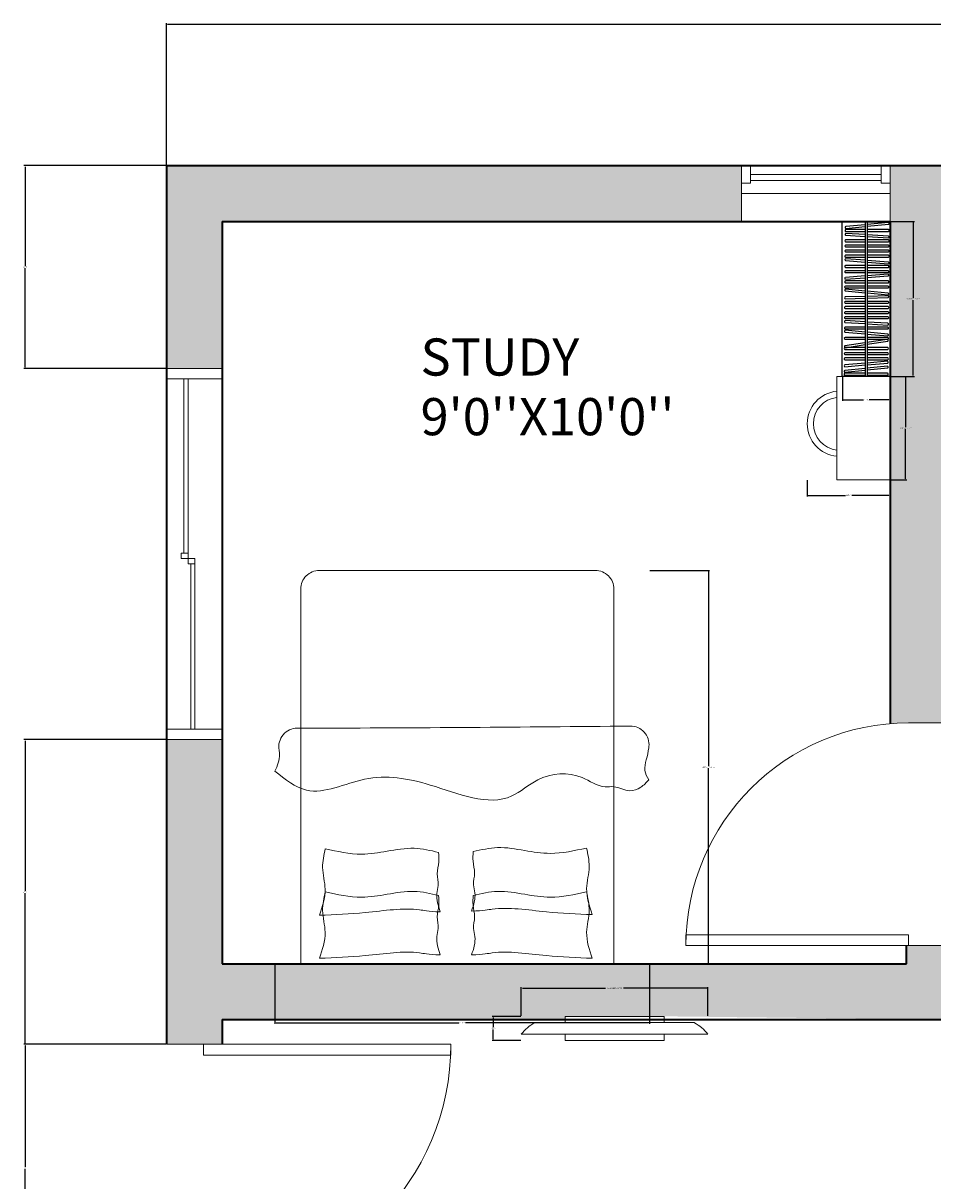
# Model space of a CAD drawing. Units: inches. Extents: x 1789 to 2841, y 3180 to 3702.
# Tile 12 of 14: x 2374 to 2521, y 3491 to 3678. Entities that reach past the tile are written whole.
import ezdxf

# ---------------------------------------------------------------- set-up
doc = ezdxf.new("R2010")
doc.units = ezdxf.units.IN
doc.header["$MEASUREMENT"] = 0
for name, color, linetype, lineweight in [('A-ANNO-DIMS', 2, 'Continuous', 18), ('A-AREA-IDEN', 7, 'Continuous', 18), ('A-EQPM', 8, 'Continuous', 18), ('A-FLOR-CASE', 34, 'Continuous', 25), ('A-WALL', 40, 'Continuous', 35), ('A-WALL-PATT', 252, 'Continuous', 13), ('DORS', 70, 'Continuous', 18), ('FURNITURE', 34, 'Continuous', 18), ('WINDOWS', 130, 'Continuous', 18)]:
    doc.layers.add(name, color=color, linetype=linetype, lineweight=lineweight)
doc.styles.get("Standard").update_dxf_attribs({"font": 'arial.ttf'})
doc.dimstyles.get("Standard").update_dxf_attribs({"dimtxt": 0.18, "dimasz": 0.18, "dimexe": 0.18, "dimexo": 0.0625, "dimgap": 0.09, "dimtad": 0, "dimtih": 1, "dimtoh": 1, "dimdec": 0, "dimzin": 0, "dimdsep": 46, "dimlunit": 3, "dimtxsty": 'Standard', "dimcen": 0.09, "dimadec": 0, "dimazin": 0, "dimtfac": 1, "dimtdec": 0, "dimtofl": 0, "dimtmove": 0, "dimatfit": 3, "dimfxl": 1, "dimtolj": 1, "dimtzin": 0, "dimarcsym": 0})

# ---------------------------------------------------------------- blocks, each defined once
blk = doc.blocks.new('HY')
for p, q in [((2053.67, 3653.75), (2074.8, 3653.75)), ((2053.67, 3652.75), (2074.8, 3652.75)), ((2052.23, 3650.66), (2076.23, 3650.66))]:
    blk.add_line(p, q)
for points in [[(2076.23, 3646.16), (2052.23, 3646.16), (2052.23, 3655.16), (2076.23, 3655.16)], [(2052.23, 3655.16), (2053.67, 3655.16), (2053.67, 3652.35), (2052.23, 3652.35)], [(2076.23, 3655.16), (2074.8, 3655.16), (2074.8, 3652.35), (2076.23, 3652.35)]]:
    blk.add_lwpolyline(points, close=True)
blk = doc.blocks.new('HYJ')
for p, q in [((2236.02, 3650.77), (2262.74, 3650.77)), ((2206.12, 3649.67), (2234.3, 3649.67)), ((2206.12, 3649), (2234.3, 3649)), ((2236.02, 3650.11), (2262.74, 3650.11))]:
    blk.add_line(p, q)
for points in [[(2204.43, 3646.16), (2264.43, 3646.16), (2264.43, 3655.16), (2204.43, 3655.16)], [(2204.43, 3655.16), (2206.12, 3655.16), (2206.12, 3646.16), (2204.43, 3646.16)], [(2264.43, 3655.16), (2262.74, 3655.16), (2262.74, 3646.16), (2264.43, 3646.16)], [(2235.16, 3650.77), (2236.02, 3650.77), (2236.02, 3649.67), (2235.16, 3649.67)], [(2234.3, 3649.67), (2235.16, 3649.67), (2235.16, 3648.56), (2234.3, 3648.56)]]:
    blk.add_lwpolyline(points, close=True)
blk = doc.blocks.new('CUBOARD')
for p, q in [((2183.73, 3646.16), (2183.73, 3568.16)), ((2184.71, 3646.16), (2184.71, 3568.16))]:
    blk.add_line(p, q)
blk.add_lwpolyline([(2172.23, 3646.16), (2196.23, 3646.16), (2196.23, 3568.16), (2172.23, 3568.16)], close=True)
for points in [[(2183.69, 3644.46), (2173.95, 3643.51)], [(2173.97, 3642.61), (2183.78, 3643.57)], [(2195.39, 3645.6), (2184.67, 3644.55)], [(2184.76, 3643.66), (2195.54, 3644.71)], [(2195.78, 3645.16), (2195.78, 3645.18)], [(2173.84, 3639.19), (2183.7, 3638.57)], [(2173.86, 3641.08), (2183.73, 3641.08)], [(2183.73, 3641.98), (2173.93, 3641.98)], [(2183.76, 3639.46), (2173.96, 3640.08)], [(2184.68, 3638.5), (2195.46, 3637.81)], [(2195.47, 3641.98), (2184.71, 3641.98)], [(2184.71, 3641.08), (2195.53, 3641.08)], [(2195.45, 3638.71), (2184.74, 3639.4)], [(2195.77, 3638.22), (2195.78, 3638.24)], [(2195.82, 3641.5), (2195.82, 3641.53)], [(2173.81, 3633.34), (2183.73, 3633.34)], [(2173.83, 3635.92), (2183.73, 3635.92)], [(2183.73, 3634.24), (2173.88, 3634.24)], [(2183.73, 3636.82), (2173.9, 3636.82)], [(2195.43, 3636.82), (2184.71, 3636.82)], [(2184.71, 3635.92), (2195.5, 3635.92)], [(2195.42, 3634.24), (2184.71, 3634.24)], [(2184.71, 3633.34), (2195.48, 3633.34)], [(2195.77, 3633.77), (2195.77, 3633.79)], [(2195.78, 3636.35), (2195.78, 3636.37)], [(2173.78, 3628.19), (2183.73, 3628.19)], [(2173.79, 3626.43), (2183.74, 3625.68)], [(2173.8, 3630.76), (2183.73, 3630.76)], [(2183.73, 3629.08), (2173.85, 3629.08)], [(2183.73, 3631.66), (2173.86, 3631.66)], [(2183.8, 3626.57), (2173.93, 3627.31)], [(2195.4, 3631.66), (2184.71, 3631.66)], [(2184.71, 3630.76), (2195.47, 3630.76)], [(2195.38, 3629.08), (2184.71, 3629.08)], [(2184.71, 3628.19), (2195.45, 3628.19)], [(2195.4, 3625.7), (2184.78, 3626.5)], [(2195.73, 3628.61), (2195.73, 3628.63)], [(2195.75, 3631.19), (2195.75, 3631.21)], [(2173.73, 3620.45), (2183.73, 3620.45)], [(2173.75, 3623.03), (2183.73, 3623.03)], [(2183.73, 3621.34), (2173.8, 3621.34)], [(2183.73, 3623.92), (2173.81, 3623.92)], [(2184.71, 3625.61), (2195.4, 3624.81)], [(2195.35, 3623.92), (2184.71, 3623.92)], [(2184.71, 3623.03), (2195.42, 3623.03)], [(2195.33, 3621.34), (2184.71, 3621.34)], [(2184.71, 3620.45), (2195.4, 3620.45)], [(2195.68, 3620.87), (2195.68, 3620.9)], [(2195.7, 3623.45), (2195.7, 3623.48)], [(2195.72, 3625.21), (2195.72, 3625.23)], [(2173.7, 3615.29), (2183.73, 3615.29)], [(2183.67, 3618.69), (2173.75, 3617.93)], [(2173.75, 3617.03), (2183.74, 3617.8)], [(2183.73, 3616.19), (2173.77, 3616.19)], [(2195.22, 3619.57), (2184.65, 3618.76)], [(2184.71, 3617.87), (2195.35, 3618.68)], [(2195.3, 3616.19), (2184.71, 3616.19)], [(2184.71, 3615.29), (2195.37, 3615.29)], [(2195.6, 3619.13), (2195.6, 3619.15)], [(2195.65, 3615.71), (2195.65, 3615.74)], [(2173.67, 3611.18), (2183.69, 3610.23)], [(2173.68, 3612.71), (2183.73, 3612.71)], [(2183.73, 3613.61), (2173.75, 3613.61)], [(2183.78, 3611.12), (2173.82, 3612.07)], [(2184.67, 3610.14), (2195.24, 3609.13)], [(2195.23, 3608.76), (2184.7, 3608.45)], [(2195.28, 3613.61), (2184.71, 3613.61)], [(2184.71, 3612.71), (2195.35, 3612.71)], [(2195.26, 3610.03), (2184.75, 3611.03)], [(2195.56, 3609.53), (2195.57, 3609.55)], [(2195.63, 3613.14), (2195.63, 3613.16)], [(2173.63, 3604.98), (2183.73, 3604.98)], [(2173.66, 3607.23), (2183.75, 3607.53)], [(2183.73, 3603.29), (2173.68, 3603.29)], [(2183.73, 3605.87), (2173.7, 3605.87)], [(2183.72, 3608.42), (2173.71, 3608.13)], [(2195.23, 3605.87), (2184.71, 3605.87)], [(2184.71, 3604.98), (2195.3, 3604.98)], [(2195.22, 3603.29), (2184.71, 3603.29)], [(2184.73, 3607.55), (2195.33, 3607.87)], [(2195.57, 3602.82), (2195.57, 3602.84)], [(2195.58, 3605.4), (2195.58, 3605.42)], [(2195.6, 3608.3), (2195.6, 3608.32)], [(2173.58, 3597.24), (2183.73, 3597.24)], [(2173.6, 3599.82), (2183.73, 3599.82)], [(2173.61, 3602.4), (2183.73, 3602.4)], [(2183.73, 3598.13), (2173.65, 3598.13)], [(2183.73, 3600.71), (2173.67, 3600.71)], [(2184.71, 3602.4), (2195.28, 3602.4)], [(2195.2, 3600.71), (2184.71, 3600.71)], [(2184.71, 3599.82), (2195.27, 3599.82)], [(2195.18, 3598.13), (2184.71, 3598.13)], [(2184.71, 3597.24), (2195.25, 3597.24)], [(2195.53, 3597.66), (2195.53, 3597.69)], [(2195.55, 3600.24), (2195.55, 3600.27)], [(2173.55, 3592.08), (2183.73, 3592.08)], [(2173.56, 3595.36), (2183.71, 3594.72)], [(2183.73, 3592.98), (2173.62, 3592.98)], [(2183.77, 3595.62), (2173.68, 3596.25)], [(2183.73, 3590.49), (2173.72, 3591.37)], [(2184.69, 3594.66), (2195.19, 3594)], [(2195.15, 3592.98), (2184.71, 3592.98)], [(2184.71, 3592.08), (2195.22, 3592.08)], [(2195.18, 3594.9), (2184.74, 3595.55)], [(2195.5, 3594.4), (2195.5, 3594.43)], [(2195.5, 3592.5), (2195.5, 3592.53)], [(2173.51, 3586.92), (2183.73, 3586.92)], [(2173.57, 3590.49), (2183.74, 3589.59)], [(2183.73, 3587.82), (2173.58, 3587.82)], [(2194.84, 3586.83), (2184.58, 3585.23)], [(2195.17, 3589.47), (2184.71, 3590.4)], [(2184.71, 3589.5), (2195.16, 3588.58)], [(2195.12, 3587.82), (2184.71, 3587.82)], [(2184.71, 3586.92), (2195.19, 3586.92)], [(2184.71, 3584.34), (2195.04, 3585.95)], [(2195.26, 3586.41), (2195.25, 3586.44)], [(2195.47, 3587.35), (2195.47, 3587.37)], [(2195.48, 3588.97), (2195.48, 3589)], [(2173.48, 3581.77), (2183.73, 3581.77)], [(2183.73, 3580.08), (2173.53, 3580.08)], [(2183.73, 3582.66), (2173.55, 3582.66)], [(2183.61, 3585.08), (2173.56, 3583.51)], [(2173.63, 3582.62), (2183.75, 3584.19)], [(2195.08, 3582.66), (2184.71, 3582.66)], [(2184.71, 3581.77), (2195.15, 3581.77)], [(2195.07, 3580.08), (2184.71, 3580.08)], [(2195.42, 3579.61), (2195.42, 3579.63)], [(2195.43, 3582.19), (2195.43, 3582.21)], [(2173.45, 3576.61), (2183.73, 3576.61)], [(2173.46, 3579.19), (2183.73, 3579.19)], [(2183.66, 3574.84), (2173.46, 3573.95)], [(2173.47, 3573.05), (2183.74, 3573.94)], [(2183.73, 3577.5), (2173.52, 3577.5)], [(2194.92, 3575.81), (2184.64, 3574.92)], [(2184.71, 3579.19), (2195.14, 3579.19)], [(2195.05, 3577.5), (2184.71, 3577.5)], [(2184.71, 3576.61), (2195.12, 3576.61)], [(2184.71, 3574.03), (2195.06, 3574.93)], [(2195.31, 3575.37), (2195.31, 3575.4)], [(2195.4, 3577.03), (2195.4, 3577.05)], [(2173.4, 3568.87), (2183.73, 3568.87)], [(2183.65, 3572.24), (2173.45, 3571.25)], [(2173.47, 3570.35), (2183.74, 3571.35)], [(2183.73, 3569.77), (2173.47, 3569.77)], [(2194.88, 3573.34), (2184.63, 3572.34)], [(2184.71, 3571.45), (2195.04, 3572.46)], [(2195, 3569.77), (2184.71, 3569.77)], [(2184.71, 3568.87), (2195.07, 3568.87)], [(2195.28, 3572.91), (2195.27, 3572.93)], [(2195.35, 3569.29), (2195.35, 3569.32)]]:
    blk.add_lwpolyline(points)
for centre, start, end in [((2195.31, 3645.13), 7.01951, 80.38602), ((2195.31, 3645.13), 299.46399, 4.10318), ((2174.06, 3641.52), 105.17532, 246.09736), ((2174.06, 3639.62), 101.52321, 242.44524), ((2174.12, 3643.06), 110.73666, 251.6587), ((2195.3, 3638.26), 357.80605, 71.17257), ((2195.3, 3638.26), 290.25053, 354.88972), ((2195.34, 3641.52), 1.45817, 74.82468), ((2195.34, 3641.52), 293.90264, 358.54183), ((2174.01, 3633.78), 105.17532, 246.09736), ((2174.02, 3636.36), 105.17532, 246.09736), ((2195.29, 3633.78), 1.45817, 74.82468), ((2195.31, 3636.36), 1.45817, 74.82468), ((2195.29, 3633.78), 293.90264, 358.54183), ((2195.31, 3636.36), 293.90264, 358.54183), ((2173.97, 3628.62), 105.17532, 246.09736), ((2173.99, 3631.2), 105.17532, 246.09736), ((2174.02, 3626.85), 100.88801, 241.81004), ((2195.26, 3628.62), 1.45817, 74.82468), ((2195.27, 3631.2), 1.45817, 74.82468), ((2195.26, 3628.62), 293.90264, 358.54183), ((2195.27, 3631.2), 293.90264, 358.54183), ((2173.92, 3620.88), 105.17532, 246.09736), ((2173.94, 3623.46), 105.17532, 246.09736), ((2195.21, 3620.88), 1.45817, 74.82468), ((2195.22, 3623.46), 1.45817, 74.82468), ((2195.24, 3625.25), 357.17085, 70.53736), ((2195.24, 3625.25), 289.61533, 354.25452), ((2195.21, 3620.88), 293.90264, 358.54183), ((2195.22, 3623.46), 293.90264, 358.54183), ((2173.89, 3615.73), 105.17532, 246.09736), ((2173.9, 3617.48), 109.55405, 250.47609), ((2195.13, 3619.1), 5.8369, 79.20341), ((2195.17, 3615.73), 1.45817, 74.82468), ((2195.13, 3619.1), 298.28138, 2.92057), ((2195.17, 3615.73), 293.90264, 358.54183), ((2173.87, 3613.15), 105.17532, 246.09736), ((2173.9, 3611.6), 99.74791, 240.66994), ((2195.12, 3608.3), 3.14082, 76.50733), ((2195.09, 3609.58), 288.47523, 353.11442), ((2195.09, 3609.58), 356.03075, 69.39726), ((2195.16, 3613.15), 1.45817, 74.82468), ((2195.16, 3613.15), 293.90264, 358.54183), ((2173.81, 3602.83), 105.17532, 246.09736), ((2173.82, 3605.41), 105.17532, 246.09736), ((2173.84, 3607.67), 106.85798, 247.78001), ((2195.09, 3602.83), 1.45817, 74.82468), ((2195.11, 3605.41), 1.45817, 74.82468), ((2195.09, 3602.83), 293.90264, 358.54183), ((2195.11, 3605.41), 293.90264, 358.54183), ((2195.12, 3608.3), 295.5853, 0.22449), ((2173.77, 3597.67), 105.17532, 246.09736), ((2173.79, 3600.25), 105.17532, 246.09736), ((2195.06, 3597.67), 1.45817, 74.82468), ((2195.08, 3600.25), 1.45817, 74.82468), ((2195.06, 3597.67), 293.90264, 358.54183), ((2195.08, 3600.25), 293.90264, 358.54183), ((2173.74, 3592.52), 105.17532, 246.09736), ((2173.78, 3595.78), 101.56602, 242.48805), ((2173.8, 3590.9), 100.11619, 241.03822), ((2195.03, 3592.52), 1.45817, 74.82468), ((2195.02, 3594.44), 357.84886, 71.21538), ((2195.02, 3594.44), 290.29334, 354.93253), ((2195.03, 3592.52), 293.90264, 358.54183), ((2173.71, 3587.36), 105.17532, 246.09736), ((2194.79, 3586.35), 10.30626, 83.67278), ((2194.79, 3586.35), 302.75074, 7.38993), ((2194.99, 3587.36), 1.45817, 74.82468), ((2195.01, 3589.03), 288.84351, 353.4827), ((2195.01, 3589.03), 356.39903, 69.76554), ((2194.99, 3587.36), 293.90264, 358.54183), ((2173.66, 3579.62), 105.17532, 246.09736), ((2173.67, 3582.2), 105.17532, 246.09736), ((2173.75, 3583.08), 114.02342, 254.94545), ((2194.94, 3579.62), 1.45817, 74.82468), ((2194.96, 3582.2), 1.45817, 74.82468), ((2194.94, 3579.62), 293.90264, 358.54183), ((2194.96, 3582.2), 293.90264, 358.54183), ((2173.63, 3573.5), 110.13137, 251.0534), ((2173.64, 3577.04), 105.17532, 246.09736), ((2194.83, 3575.34), 6.41421, 79.78072), ((2194.93, 3577.04), 1.45817, 74.82468), ((2194.83, 3575.34), 298.85869, 3.49788), ((2194.93, 3577.04), 293.90264, 358.54183), ((2173.59, 3569.31), 105.17532, 246.09736), ((2173.62, 3570.8), 110.7648, 251.68684), ((2194.8, 3572.87), 7.04765, 80.41416), ((2194.88, 3569.31), 1.45817, 74.82468), ((2194.8, 3572.87), 299.49213, 4.13132), ((2194.88, 3569.31), 293.90264, 358.54183)]:
    blk.add_arc(centre, 0.476, start, end)
blk = doc.blocks.new('KIKI')
blk.add_lwpolyline([(2076.23, 3621.09), (2067.63, 3621.09), (2067.63, 3604.37), (2076.23, 3604.37)], close=True)
for radius, start, end in [(5.28, 95.3029, 264.6971), (4.28, 96.5454, 263.4546)]:
    blk.add_arc((2068.12, 3613.45), radius, start, end)
blk = doc.blocks.new('BED')
blk.add_lwpolyline([(1986.04, 3526.16), (2036.66, 3526.16), (2036.66, 3586.73, 0.414214), (2033.66, 3589.73), (1989.04, 3589.73, 0.414214), (1986.04, 3586.73)], format="xyb", close=True)
for centre, start, end in [((2039.35, 3561.59), 353.8505, 90.5407), ((1985.49, 3561.26), 90.0009, 190.5913)]:
    blk.add_arc(centre, 3, start, end)
for points, knots in [([(1985.49, 3564.26), (1986.18, 3564.26), (2004.12, 3564.26), (2022.07, 3564.42), (2039.32, 3564.59)], [3.01567, 3.01567, 3.01567, 3.01567, 5.086115, 56.845422, 56.845422, 56.845422, 56.845422]), ([(1981.86, 3557.29), (1982.25, 3558.19), (1982.74, 3559.32), (1982.58, 3560.48), (1982.54, 3560.71)], [0, 0, 0, 0, 2.832176, 3.533558, 3.533558, 3.533558, 3.533558]), ([(2042.33, 3561.27), (2042.32, 3561.2), (2042.24, 3560.49), (2041.94, 3559.24), (2041.44, 3557.42), (2042.02, 3556.4), (2042.31, 3555.9)], [3.346066, 3.346066, 3.346066, 3.346066, 3.533964, 5.519604, 7.243879, 8.905148, 8.905148, 8.905148, 8.905148]), ([(1981.86, 3557.29), (1983.51, 3555.96), (1987.81, 3552.49), (1996.85, 3557.26), (2007.63, 3555.42), (2018.15, 3550.73), (2024.7, 3556.86), (2030.75, 3557.33), (2034.33, 3554.54), (2037.1, 3554.97), (2038.94, 3553.79), (2041.09, 3554.56), (2041.91, 3555.46), (2042.31, 3555.9)], [0, 0, 0, 0, 5.964303, 15.522281, 26.165437, 39.489609, 44.417923, 51.588888, 55.595283, 57.020157, 59.675402, 61.528396, 63.30469, 63.30469, 63.30469, 63.30469]), ([(1989.08, 3534), (1989.54, 3535.4), (1990.39, 3537.95), (1989.29, 3541.59), (1989.78, 3543.76), (1990, 3544.76)], [0, 0, 0, 0, 4.309756, 7.868817, 10.904955, 10.904955, 10.904955, 10.904955]), ([(1990, 3544.76), (1991.96, 3544.32), (1995.28, 3543.58), (2000.08, 3544.36), (2004.25, 3545.12), (2007.01, 3544.48), (2008.32, 3544.17)], [0, 0, 0, 0, 5.938346, 10.092725, 14.493934, 18.489388, 18.489388, 18.489388, 18.489388]), ([(2008.32, 3544.17), (2008.36, 3543.66), (2008.45, 3542.49), (2007.91, 3540.73), (2008.43, 3539.01), (2007.78, 3536.97), (2008.25, 3535.55), (2008.59, 3534.55)], [0, 0, 0, 0, 1.551238, 3.49035, 5.35792, 6.678685, 9.712273, 9.712273, 9.712273, 9.712273]), ([(2013.92, 3544.29), (2013.88, 3543.77), (2013.79, 3542.61), (2014.33, 3540.84), (2013.81, 3539.13), (2014.46, 3537.09), (2013.99, 3535.66), (2013.65, 3534.67)], [0, 0, 0, 0, 1.551238, 3.49035, 5.35792, 6.678685, 9.712273, 9.712273, 9.712273, 9.712273]), ([(2032.24, 3544.88), (2030.28, 3544.44), (2026.96, 3543.7), (2022.16, 3544.48), (2017.99, 3545.23), (2015.23, 3544.59), (2013.92, 3544.29)], [0, 0, 0, 0, 5.938346, 10.092725, 14.493934, 18.489388, 18.489388, 18.489388, 18.489388]), ([(2033.16, 3534.12), (2032.7, 3535.52), (2031.85, 3538.07), (2032.95, 3541.7), (2032.46, 3543.88), (2032.24, 3544.88)], [0, 0, 0, 0, 4.309756, 7.868817, 10.904955, 10.904955, 10.904955, 10.904955]), ([(1989.08, 3527.05), (1989.54, 3528.44), (1990.39, 3531), (1989.29, 3534.63), (1989.78, 3536.8), (1990, 3537.8)], [0, 0, 0, 0, 4.309756, 7.868817, 10.904955, 10.904955, 10.904955, 10.904955]), ([(1990, 3537.8), (1991.96, 3537.37), (1995.28, 3536.62), (2000.08, 3537.4), (2004.25, 3538.16), (2007.01, 3537.52), (2008.32, 3537.22)], [0, 0, 0, 0, 5.938346, 10.092725, 14.493934, 18.489388, 18.489388, 18.489388, 18.489388]), ([(2008.32, 3537.22), (2008.36, 3536.7), (2008.45, 3535.53), (2007.91, 3533.77), (2008.43, 3532.06), (2007.78, 3530.02), (2008.25, 3528.59), (2008.59, 3527.59)], [0, 0, 0, 0, 1.551238, 3.49035, 5.35792, 6.678685, 9.712273, 9.712273, 9.712273, 9.712273]), ([(2013.92, 3537.22), (2013.88, 3536.7), (2013.79, 3535.53), (2014.33, 3533.77), (2013.81, 3532.06), (2014.46, 3530.02), (2013.99, 3528.59), (2013.65, 3527.59)], [0, 0, 0, 0, 1.551238, 3.49035, 5.35792, 6.678685, 9.712273, 9.712273, 9.712273, 9.712273]), ([(2032.24, 3537.8), (2030.28, 3537.37), (2026.96, 3536.62), (2022.16, 3537.4), (2017.99, 3538.16), (2015.23, 3537.52), (2013.92, 3537.22)], [0, 0, 0, 0, 5.938346, 10.092725, 14.493934, 18.489388, 18.489388, 18.489388, 18.489388]), ([(2033.16, 3527.05), (2032.7, 3528.44), (2031.85, 3531), (2032.95, 3534.63), (2032.46, 3536.8), (2032.24, 3537.8)], [0, 0, 0, 0, 4.309756, 7.868817, 10.904955, 10.904955, 10.904955, 10.904955]), ([(1989.08, 3534), (1991.55, 3534.11), (1997.16, 3534.35), (2003.38, 3535.37), (2006.53, 3534.65), (2008.59, 3534.55)], [0, 0, 0, 0, 7.448152, 16.876341, 19.223863, 19.223863, 19.223863, 19.223863]), ([(2033.16, 3534.12), (2030.69, 3534.22), (2025.08, 3534.46), (2018.86, 3535.49), (2015.71, 3534.77), (2013.65, 3534.67)], [0, 0, 0, 0, 7.448152, 16.876341, 19.223863, 19.223863, 19.223863, 19.223863]), ([(1989.08, 3527.05), (1991.55, 3527.15), (1997.16, 3527.39), (2003.38, 3528.41), (2006.53, 3527.69), (2008.59, 3527.59)], [0, 0, 0, 0, 7.448152, 16.876341, 19.223863, 19.223863, 19.223863, 19.223863]), ([(2033.16, 3527.05), (2030.69, 3527.15), (2025.08, 3527.39), (2018.86, 3528.41), (2015.71, 3527.69), (2013.65, 3527.59)], [0, 0, 0, 0, 7.448152, 16.876341, 19.223863, 19.223863, 19.223863, 19.223863])]:
    blk.add_open_spline(points, degree=3, knots=knots)
blk = doc.blocks.new('*U9')
for p, q in [((0, 0), (0, -6)), ((36, 0), (36, -6))]:
    blk.add_line(p, q)
blk.add_lwpolyline([(0, 0), (0, 36), (1.75, 36), (1.75, 0)], close=True)
blk.add_arc((0, 0), 36, 0, 90)
blk = doc.blocks.new('GTGTG')
for points in [[(2261.92, 3645.14), (2287.72, 3645.14)], [(2289.9, 3643.29), (2259.74, 3643.29)]]:
    blk.add_lwpolyline(points)
for points in [[(2266.82, 3646.16), (2282.82, 3646.16), (2282.82, 3645.14), (2266.82, 3645.14)], [(2266.82, 3643.29), (2282.82, 3643.29), (2282.82, 3642.27), (2266.82, 3642.27)]]:
    blk.add_lwpolyline(points, close=True)
for centre, start, end in [((2265.21, 3639.05), 118.4184, 142.2436), ((2284.43, 3639.05), 37.7564, 61.5816)]:
    blk.add_arc(centre, 6.92, start, end)
blk = doc.blocks.new('*U26')
for p, q in [((0, 0), (0, -6)), ((40, 0), (40, -6))]:
    blk.add_line(p, q)
blk.add_lwpolyline([(0, 0), (0, 40), (1.75, 40), (1.75, 0)], close=True)
blk.add_arc((0, 0), 40, 0, 90)
blk = doc.blocks.new('*D39')
at = {"layer": 'A-ANNO-DIMS', "color": 0, "lineweight": -2, "transparency": 16777216}
for p, q in [((2514.3, 3646.16), (2518.17, 3646.16)), ((2517.99, 3645.98), (2517.99, 3633.81)), ((2517.99, 3621.27), (2517.99, 3633.44)), ((2514.3, 3621.09), (2518.17, 3621.09))]:
    blk.add_line(p, q, dxfattribs=at)
at = {"layer": 'A-ANNO-DIMS', "color": 0, "transparency": 16777216}
for points in [[(2517.96, 3645.98), (2518.02, 3645.98), (2517.99, 3646.16)], [(2517.96, 3621.27), (2518.02, 3621.27), (2517.99, 3621.09)]]:
    blk.add_solid(points, dxfattribs=at)
at = {"layer": 'Defpoints', "color": 0, "transparency": 16777216}
for p in [(2514.23, 3646.16), (2517.99, 3646.16), (2514.23, 3621.09)]:
    blk.add_point(p, dxfattribs=at)
at = {"layer": 'A-ANNO-DIMS', "color": 0, "transparency": 16777216, "insert": (2517.99, 3633.62), "char_height": 0.18, "attachment_point": 5}
blk.add_mtext('\\A1;WARDROBE 25 TYP.', dxfattribs=at)
blk = doc.blocks.new('*D40')
at = {"layer": 'A-ANNO-DIMS', "color": 0, "lineweight": -2, "transparency": 16777216}
for p, q in [((2506.52, 3621.02), (2506.52, 3617.15)), ((2514.23, 3621.02), (2514.23, 3617.15)), ((2506.7, 3617.33), (2509.92, 3617.33)), ((2514.05, 3617.33), (2510.83, 3617.33))]:
    blk.add_line(p, q, dxfattribs=at)
at = {"layer": 'A-ANNO-DIMS', "color": 0, "transparency": 16777216}
for points in [[(2506.7, 3617.36), (2506.7, 3617.3), (2506.52, 3617.33)], [(2514.05, 3617.36), (2514.05, 3617.3), (2514.23, 3617.33)]]:
    blk.add_solid(points, dxfattribs=at)
at = {"layer": 'Defpoints', "color": 0, "transparency": 16777216}
for p in [(2506.52, 3621.09), (2514.23, 3621.09), (2514.23, 3617.33)]:
    blk.add_point(p, dxfattribs=at)
at = {"layer": 'A-ANNO-DIMS', "color": 0, "transparency": 16777216, "insert": (2510.38, 3617.33), "char_height": 0.18, "attachment_point": 5}
blk.add_mtext('\\A1;8 TYP.', dxfattribs=at)
blk = doc.blocks.new('*D41')
at = {"layer": 'A-ANNO-DIMS', "color": 0, "lineweight": -2, "transparency": 16777216}
for p, q in [((2454.61, 3517.73), (2454.61, 3522.38)), ((2454.79, 3522.2), (2468.22, 3522.2)), ((2484.59, 3522.2), (2471.16, 3522.2)), ((2484.77, 3517.73), (2484.77, 3522.38))]:
    blk.add_line(p, q, dxfattribs=at)
at = {"layer": 'A-ANNO-DIMS', "color": 0, "transparency": 16777216}
for points in [[(2454.79, 3522.23), (2454.79, 3522.17), (2454.61, 3522.2)], [(2484.59, 3522.23), (2484.59, 3522.17), (2484.77, 3522.2)]]:
    blk.add_solid(points, dxfattribs=at)
at = {"layer": 'Defpoints', "color": 0, "transparency": 16777216}
for p in [(2484.77, 3522.2), (2454.61, 3517.67), (2484.77, 3517.67)]:
    blk.add_point(p, dxfattribs=at)
at = {"layer": 'A-ANNO-DIMS', "color": 0, "transparency": 16777216, "insert": (2469.69, 3522.2), "char_height": 0.18, "attachment_point": 5}
blk.add_mtext('\\A1;WALL SCREEN 30 TYP.', dxfattribs=at)
blk = doc.blocks.new('*D42')
at = {"layer": 'A-ANNO-DIMS', "color": 0, "lineweight": -2, "transparency": 16777216}
for p, q in [((2454.55, 3517.67), (2449.91, 3517.67)), ((2450.09, 3517.49), (2450.09, 3515.91)), ((2450.09, 3513.96), (2450.09, 3515.54)), ((2454.55, 3513.78), (2449.91, 3513.78))]:
    blk.add_line(p, q, dxfattribs=at)
at = {"layer": 'A-ANNO-DIMS', "color": 0, "transparency": 16777216}
for points in [[(2450.06, 3517.49), (2450.12, 3517.49), (2450.09, 3517.67)], [(2450.06, 3513.96), (2450.12, 3513.96), (2450.09, 3513.78)]]:
    blk.add_solid(points, dxfattribs=at)
at = {"layer": 'Defpoints', "color": 0, "transparency": 16777216}
for p in [(2450.09, 3517.67), (2454.61, 3517.67), (2454.61, 3513.78)]:
    blk.add_point(p, dxfattribs=at)
at = {"layer": 'A-ANNO-DIMS', "color": 0, "transparency": 16777216, "insert": (2450.09, 3515.73), "char_height": 0.18, "attachment_point": 5}
blk.add_mtext('\\A1;4 TYP.', dxfattribs=at)
blk = doc.blocks.new('*D47')
at = {"layer": 'A-ANNO-DIMS', "color": 0, "lineweight": -2, "transparency": 16777216}
for p, q in [((2514.3, 3621.09), (2516.92, 3621.09)), ((2516.74, 3620.91), (2516.74, 3612.91)), ((2516.74, 3604.55), (2516.74, 3612.55)), ((2514.3, 3604.37), (2516.92, 3604.37))]:
    blk.add_line(p, q, dxfattribs=at)
at = {"layer": 'A-ANNO-DIMS', "color": 0, "transparency": 16777216}
for points in [[(2516.71, 3620.91), (2516.77, 3620.91), (2516.74, 3621.09)], [(2516.71, 3604.55), (2516.77, 3604.55), (2516.74, 3604.37)]]:
    blk.add_solid(points, dxfattribs=at)
at = {"layer": 'Defpoints', "color": 0, "transparency": 16777216}
for p in [(2514.23, 3621.09), (2516.74, 3621.09), (2514.23, 3604.37)]:
    blk.add_point(p, dxfattribs=at)
at = {"layer": 'A-ANNO-DIMS', "color": 0, "transparency": 16777216, "insert": (2516.74, 3612.73), "char_height": 0.18, "attachment_point": 5}
blk.add_mtext('\\A1;DESK SET 17 TYP.', dxfattribs=at)
blk = doc.blocks.new('*D48')
at = {"layer": 'A-ANNO-DIMS', "color": 0, "lineweight": -2, "transparency": 16777216}
for p, q in [((2500.83, 3604.31), (2500.83, 3601.69)), ((2514.23, 3604.31), (2514.23, 3601.69)), ((2501.01, 3601.87), (2507.01, 3601.87)), ((2514.05, 3601.87), (2508.05, 3601.87))]:
    blk.add_line(p, q, dxfattribs=at)
at = {"layer": 'A-ANNO-DIMS', "color": 0, "transparency": 16777216}
for points in [[(2501.01, 3601.9), (2501.01, 3601.84), (2500.83, 3601.87)], [(2514.05, 3601.9), (2514.05, 3601.84), (2514.23, 3601.87)]]:
    blk.add_solid(points, dxfattribs=at)
at = {"layer": 'Defpoints', "color": 0, "transparency": 16777216}
for p in [(2500.83, 3604.37), (2514.23, 3604.37), (2514.23, 3601.87)]:
    blk.add_point(p, dxfattribs=at)
at = {"layer": 'A-ANNO-DIMS', "color": 0, "transparency": 16777216, "insert": (2507.53, 3601.87), "char_height": 0.18, "attachment_point": 5}
blk.add_mtext('\\A1;13 TYP.', dxfattribs=at)
blk = doc.blocks.new('*D59')
at = {"layer": 'A-ANNO-DIMS', "color": 0, "lineweight": -2, "transparency": 16777216}
for p, q in [((2475.4, 3589.73), (2485.06, 3589.73)), ((2484.88, 3589.55), (2484.88, 3558.13)), ((2484.88, 3526.34), (2484.88, 3557.76)), ((2475.4, 3526.16), (2485.06, 3526.16))]:
    blk.add_line(p, q, dxfattribs=at)
at = {"layer": 'A-ANNO-DIMS', "color": 0, "transparency": 16777216}
for points in [[(2484.85, 3589.55), (2484.91, 3589.55), (2484.88, 3589.73)], [(2484.85, 3526.34), (2484.91, 3526.34), (2484.88, 3526.16)]]:
    blk.add_solid(points, dxfattribs=at)
at = {"layer": 'Defpoints', "color": 0, "transparency": 16777216}
for p in [(2475.34, 3589.73), (2484.88, 3589.73), (2475.34, 3526.16)]:
    blk.add_point(p, dxfattribs=at)
at = {"layer": 'A-ANNO-DIMS', "color": 0, "transparency": 16777216, "insert": (2484.88, 3557.95), "char_height": 0.18, "attachment_point": 5}
blk.add_mtext('\\A1;STUDY BED 64 TYP.', dxfattribs=at)
blk = doc.blocks.new('*D60')
at = {"layer": 'A-ANNO-DIMS', "color": 0, "lineweight": -2, "transparency": 16777216}
for p, q in [((2414.78, 3526.1), (2414.78, 3516.44)), ((2475.34, 3526.1), (2475.34, 3516.44)), ((2414.96, 3516.62), (2444.53, 3516.62)), ((2475.16, 3516.62), (2445.59, 3516.62))]:
    blk.add_line(p, q, dxfattribs=at)
at = {"layer": 'A-ANNO-DIMS', "color": 0, "transparency": 16777216}
for points in [[(2414.96, 3516.65), (2414.96, 3516.59), (2414.78, 3516.62)], [(2475.16, 3516.65), (2475.16, 3516.59), (2475.34, 3516.62)]]:
    blk.add_solid(points, dxfattribs=at)
at = {"layer": 'Defpoints', "color": 0, "transparency": 16777216}
for p in [(2414.78, 3526.16), (2475.34, 3526.16), (2475.34, 3516.62)]:
    blk.add_point(p, dxfattribs=at)
at = {"layer": 'A-ANNO-DIMS', "color": 0, "transparency": 16777216, "insert": (2445.06, 3516.62), "char_height": 0.18, "attachment_point": 5}
blk.add_mtext('\\A1;61 TYP.', dxfattribs=at)
blk = doc.blocks.new('*D95')
at = {"layer": 'A-ANNO-DIMS', "color": 0, "lineweight": -2, "transparency": 16777216}
for p, q in [((2397.23, 3655.22), (2397.23, 3678.19)), ((2397.41, 3678.01), (2599.44, 3678.01)), ((2802.05, 3678.01), (2600.03, 3678.01)), ((2802.23, 3526.22), (2802.23, 3678.19))]:
    blk.add_line(p, q, dxfattribs=at)
at = {"layer": 'A-ANNO-DIMS', "color": 0, "transparency": 16777216}
for points in [[(2397.41, 3678.04), (2397.41, 3677.98), (2397.23, 3678.01)], [(2802.05, 3678.04), (2802.05, 3677.98), (2802.23, 3678.01)]]:
    blk.add_solid(points, dxfattribs=at)
at = {"layer": 'Defpoints', "color": 0, "transparency": 16777216}
for p in [(2802.23, 3678.01), (2397.23, 3655.16), (2802.23, 3526.16)]:
    blk.add_point(p, dxfattribs=at)
at = {"layer": 'A-ANNO-DIMS', "color": 0, "transparency": 16777216, "insert": (2599.73, 3678.01), "char_height": 0.18, "attachment_point": 5}
blk.add_mtext('\\A1;405', dxfattribs=at)
blk = doc.blocks.new('*D102')
at = {"layer": 'A-ANNO-DIMS', "color": 0, "lineweight": -2, "transparency": 16777216}
for p, q in [((2397.17, 3655.16), (2374.2, 3655.16)), ((2374.38, 3654.98), (2374.38, 3638.96)), ((2374.38, 3622.57), (2374.38, 3638.6)), ((2397.17, 3622.39), (2374.2, 3622.39))]:
    blk.add_line(p, q, dxfattribs=at)
at = {"layer": 'A-ANNO-DIMS', "color": 0, "transparency": 16777216}
for points in [[(2374.35, 3654.98), (2374.41, 3654.98), (2374.38, 3655.16)], [(2374.35, 3622.57), (2374.41, 3622.57), (2374.38, 3622.39)]]:
    blk.add_solid(points, dxfattribs=at)
at = {"layer": 'Defpoints', "color": 0, "transparency": 16777216}
for p in [(2397.23, 3655.16), (2374.38, 3622.39), (2397.23, 3622.39)]:
    blk.add_point(p, dxfattribs=at)
at = {"layer": 'A-ANNO-DIMS', "color": 0, "transparency": 16777216, "insert": (2374.38, 3638.78), "char_height": 0.18, "attachment_point": 5}
blk.add_mtext('\\A1;32.77', dxfattribs=at)
blk = doc.blocks.new('*D103')
at = {"layer": 'A-ANNO-DIMS', "color": 0, "lineweight": -2, "transparency": 16777216}
for p, q in [((2397.17, 3562.39), (2374.2, 3562.39)), ((2374.38, 3562.21), (2374.38, 3537.96)), ((2374.38, 3513.34), (2374.38, 3537.6)), ((2397.17, 3513.16), (2374.2, 3513.16))]:
    blk.add_line(p, q, dxfattribs=at)
at = {"layer": 'A-ANNO-DIMS', "color": 0, "transparency": 16777216}
for points in [[(2374.35, 3562.21), (2374.41, 3562.21), (2374.38, 3562.39)], [(2374.35, 3513.34), (2374.41, 3513.34), (2374.38, 3513.16)]]:
    blk.add_solid(points, dxfattribs=at)
at = {"layer": 'Defpoints', "color": 0, "transparency": 16777216}
for p in [(2397.23, 3562.39), (2374.38, 3513.16), (2397.23, 3513.16)]:
    blk.add_point(p, dxfattribs=at)
at = {"layer": 'A-ANNO-DIMS', "color": 0, "transparency": 16777216, "insert": (2374.38, 3537.78), "char_height": 0.18, "attachment_point": 5}
blk.add_mtext('\\A1;49.23', dxfattribs=at)
blk = doc.blocks.new('*D104')
at = {"layer": 'A-ANNO-DIMS', "color": 0, "lineweight": -2, "transparency": 16777216}
for p, q in [((2397.17, 3513.16), (2374.2, 3513.16)), ((2374.38, 3512.98), (2374.38, 3493.34)), ((2374.38, 3473.34), (2374.38, 3492.98)), ((2397.17, 3473.16), (2374.2, 3473.16))]:
    blk.add_line(p, q, dxfattribs=at)
at = {"layer": 'A-ANNO-DIMS', "color": 0, "transparency": 16777216}
for points in [[(2374.35, 3512.98), (2374.41, 3512.98), (2374.38, 3513.16)], [(2374.35, 3473.34), (2374.41, 3473.34), (2374.38, 3473.16)]]:
    blk.add_solid(points, dxfattribs=at)
at = {"layer": 'Defpoints', "color": 0, "transparency": 16777216}
for p in [(2397.23, 3513.16), (2374.38, 3473.16), (2397.23, 3473.16)]:
    blk.add_point(p, dxfattribs=at)
at = {"layer": 'A-ANNO-DIMS', "color": 0, "transparency": 16777216, "insert": (2374.38, 3493.16), "char_height": 0.18, "attachment_point": 5}
blk.add_mtext('\\A1;40', dxfattribs=at)

msp = doc.modelspace()

# ---------------------------------------------------------------- hatches: boundary and pattern name
at = {"layer": 'A-WALL-PATT'}
h = msp.add_hatch(color=256, dxfattribs=at)
h.dxf.hatch_style = 1
h.paths.add_polyline_path([(2490.2333, 3655.1608), (2397.2333, 3655.1608), (2397.2333, 3622.3936), (2406.2333, 3622.3936), (2406.2333, 3646.1608), (2490.2333, 3646.1608)])
h.paths.add_polyline_path([(2642.4325, 3655.1608), (2555.6786, 3655.1608), (2555.6786, 3646.1608), (2601.2333, 3646.1608), (2601.2333, 3640.1475), (2601.2333, 3568.1608), (2597.2333, 3568.1608), (2597.2333, 3565.4274), (2601.2333, 3565.4274), (2601.2333, 3528.1608), (2601.2333, 3517.1608), (2612.9879, 3517.1608), (2613.0522, 3523.352), (2613.0813, 3526.1608), (2610.2333, 3526.1608), (2610.2333, 3646.1608), (2634.2333, 3646.1608), (2642.4325, 3646.1608)])
h.paths.add_polyline_path([(2523.2333, 3646.1608), (2531.6786, 3646.1608), (2531.6786, 3655.1608), (2514.2333, 3655.1608), (2514.2333, 3646.1608), (2514.2333, 3621.0865), (2514.2333, 3564.976, -0.02086055), (2517.2333, 3565.1012), (2523.2333, 3565.1012), (2523.2333, 3565.4274), (2567.2333, 3565.4274), (2567.2333, 3568.1608), (2523.2333, 3568.1608)])
h = msp.add_hatch(color=256, dxfattribs=at)
h.dxf.hatch_style = 1
h.paths.add_polyline_path([(2406.2333, 3517.1608), (2461.6918, 3517.1608), (2461.6918, 3517.6724), (2477.6863, 3517.6724), (2523.2333, 3517.1608), (2523.2333, 3529.1012), (2516.8782, 3529.1012), (2516.8782, 3526.1608), (2406.2333, 3526.1608), (2406.2333, 3562.3936), (2397.2333, 3562.3936), (2397.2333, 3513.1608), (2403.2333, 3513.1608), (2406.2333, 3513.1608)])

# ---------------------------------------------------------------- linework, layer by layer
at = {"layer": 'A-WALL'}
for p, q in [((2397.2333, 3655.1608), (2397.2333, 3562.3936)), ((2397.2333, 3655.1608), (2763.2333, 3655.1608)), ((2406.2333, 3646.1608), (2406.2333, 3526.1608)), ((2406.2333, 3646.1608), (2514.2333, 3646.1608)), ((2514.2333, 3646.1608), (2514.2333, 3564.976)), ((2397.2333, 3562.3936), (2397.2333, 3513.1608)), ((2516.8782, 3526.1608), (2516.8782, 3529.1012)), ((2406.2333, 3526.1608), (2516.8782, 3526.1608)), ((2406.2333, 3517.1608), (2523.2333, 3517.1608)), ((2406.2333, 3517.1608), (2406.2333, 3513.1608))]:
    msp.add_line(p, q, dxfattribs=at)

# ---------------------------------------------------------------- block references
at = {"layer": 'A-EQPM'}
msp.add_blockref('GTGTG', (194.8709, -128.4884), dxfattribs=at)
at = {"layer": 'A-FLOR-CASE', "xscale": 0.3214652351977254, "yscale": 0.3214652351977254, "zscale": 0.3214652351977254}
msp.add_blockref('CUBOARD', (1808.2207, 2474.0469), dxfattribs=at)
at = {"layer": 'DORS'}
for name, p, rotation in [('*U9', (2517.2333, 3529.1012), 90.00000000000003), ('*U26', (2403.2333, 3513.1608), 270)]:
    msp.add_blockref(name, p, dxfattribs=dict(at, rotation=rotation))
at = {"layer": 'FURNITURE'}
for name, p in [('KIKI', (438, 0)), ('BED', (432.9199, 0))]:
    msp.add_blockref(name, p, dxfattribs=at)
at = {"layer": 'WINDOWS'}
msp.add_blockref('HY', (438, 0), dxfattribs=at)
at = {"layer": 'WINDOWS', "rotation": 270}
msp.add_blockref('HYJ', (-1248.9274, 5826.8261), dxfattribs=at)

# ---------------------------------------------------------------- texts
at = {"layer": 'A-ANNO-DIMS'}
msp.add_text("9'0''X10'0''", height=6, dxfattribs=at).set_placement((2438.3244, 3611.5922))
at = {"layer": 'A-AREA-IDEN'}
msp.add_text('STUDY', height=6, dxfattribs=at).set_placement((2438.3244, 3621.2307))

# ---------------------------------------------------------------- dimensions: what is measured, and where the dimension line sits
at = {"layer": 'A-ANNO-DIMS'}
dim = msp.add_linear_dim(base=(2802.2333, 3678.0108), p1=(2397.2333, 3655.1608), p2=(2802.2333, 3526.1608), dimstyle='Standard', override={"dimdec": 0, "dimlfac": 1, "dimrnd": 0, "dimzin": 0, "dimdsep": 46, "dimlunit": 2}, dxfattribs=at)
dim.commit()
dim.dimension.update_dxf_attribs({"geometry": '*D95', "text_midpoint": (2599.7333, 3678.0108)})
for base, p1, p2, override, picture, middle in [((2374.3833, 3622.3936), (2397.2333, 3655.1608), (2397.2333, 3622.3936), {"dimdec": 2, "dimlfac": 1, "dimrnd": 0, "dimzin": 0, "dimdsep": 46, "dimlunit": 2}, '*D102', (2374.3833, 3638.7772)), ((2374.3833, 3513.1608), (2397.2333, 3562.3936), (2397.2333, 3513.1608), {"dimdec": 2, "dimlfac": 1, "dimrnd": 0, "dimzin": 0, "dimdsep": 46, "dimlunit": 2}, '*D103', (2374.3833, 3537.7772)), ((2374.3833, 3473.1608), (2397.2333, 3513.1608), (2397.2333, 3473.1608), {"dimdec": 0, "dimlfac": 1, "dimrnd": 0, "dimzin": 0, "dimdsep": 46, "dimlunit": 2}, '*D104', (2374.3833, 3493.1608))]:
    dim = msp.add_linear_dim(base=base, p1=p1, p2=p2, angle=90, dimstyle='Standard', override=override, dxfattribs=at)
    dim.commit()
    dim.dimension.update_dxf_attribs({"geometry": picture, "text_midpoint": middle})
for base, p1, p2, text, picture, middle in [((2517.9945, 3646.1608), (2514.2333, 3621.0865), (2514.2333, 3646.1608), 'WARDROBE <> TYP.', '*D39', (2517.9945, 3633.6236)), ((2516.7401, 3621.0865), (2514.2333, 3604.3747), (2514.2333, 3621.0865), 'DESK SET <> TYP.', '*D47', (2516.7401, 3612.7306)), ((2484.8773, 3589.7335), (2475.3414, 3526.1608), (2475.3414, 3589.7335), 'STUDY BED <> TYP.', '*D59', (2484.8773, 3557.9471)), ((2450.0868, 3517.6724), (2454.6104, 3513.7776), (2454.6104, 3517.6724), '<> TYP.', '*D42', (2450.0868, 3515.725))]:
    dim = msp.add_linear_dim(base=base, p1=p1, p2=p2, angle=90, text=text, dimstyle='Standard', override={"dimdec": 0, "dimlfac": 1, "dimrnd": 0, "dimzin": 0, "dimdsep": 46, "dimlunit": 2}, dxfattribs=at)
    dim.commit()
    dim.dimension.update_dxf_attribs({"geometry": picture, "text_midpoint": middle})
for base, p1, p2, text, picture, middle in [((2514.2333, 3617.3254), (2506.5182, 3621.0865), (2514.2333, 3621.0865), '<> TYP.', '*D40', (2510.3758, 3617.3254)), ((2514.2333, 3601.8679), (2500.8307, 3604.3747), (2514.2333, 3604.3747), '<> TYP.', '*D48', (2507.532, 3601.8679)), ((2475.3414, 3516.6249), (2414.7751, 3526.1608), (2475.3414, 3526.1608), '<> TYP.', '*D60', (2445.0583, 3516.6249)), ((2484.7676, 3522.196), (2454.6104, 3517.6724), (2484.7676, 3517.6724), 'WALL SCREEN <> TYP.', '*D41', (2469.689, 3522.196))]:
    dim = msp.add_linear_dim(base=base, p1=p1, p2=p2, text=text, dimstyle='Standard', override={"dimdec": 0, "dimlfac": 1, "dimrnd": 0, "dimzin": 0, "dimdsep": 46, "dimlunit": 2}, dxfattribs=at)
    dim.commit()
    dim.dimension.update_dxf_attribs({"geometry": picture, "text_midpoint": middle})

doc.saveas('drawing.dxf')
